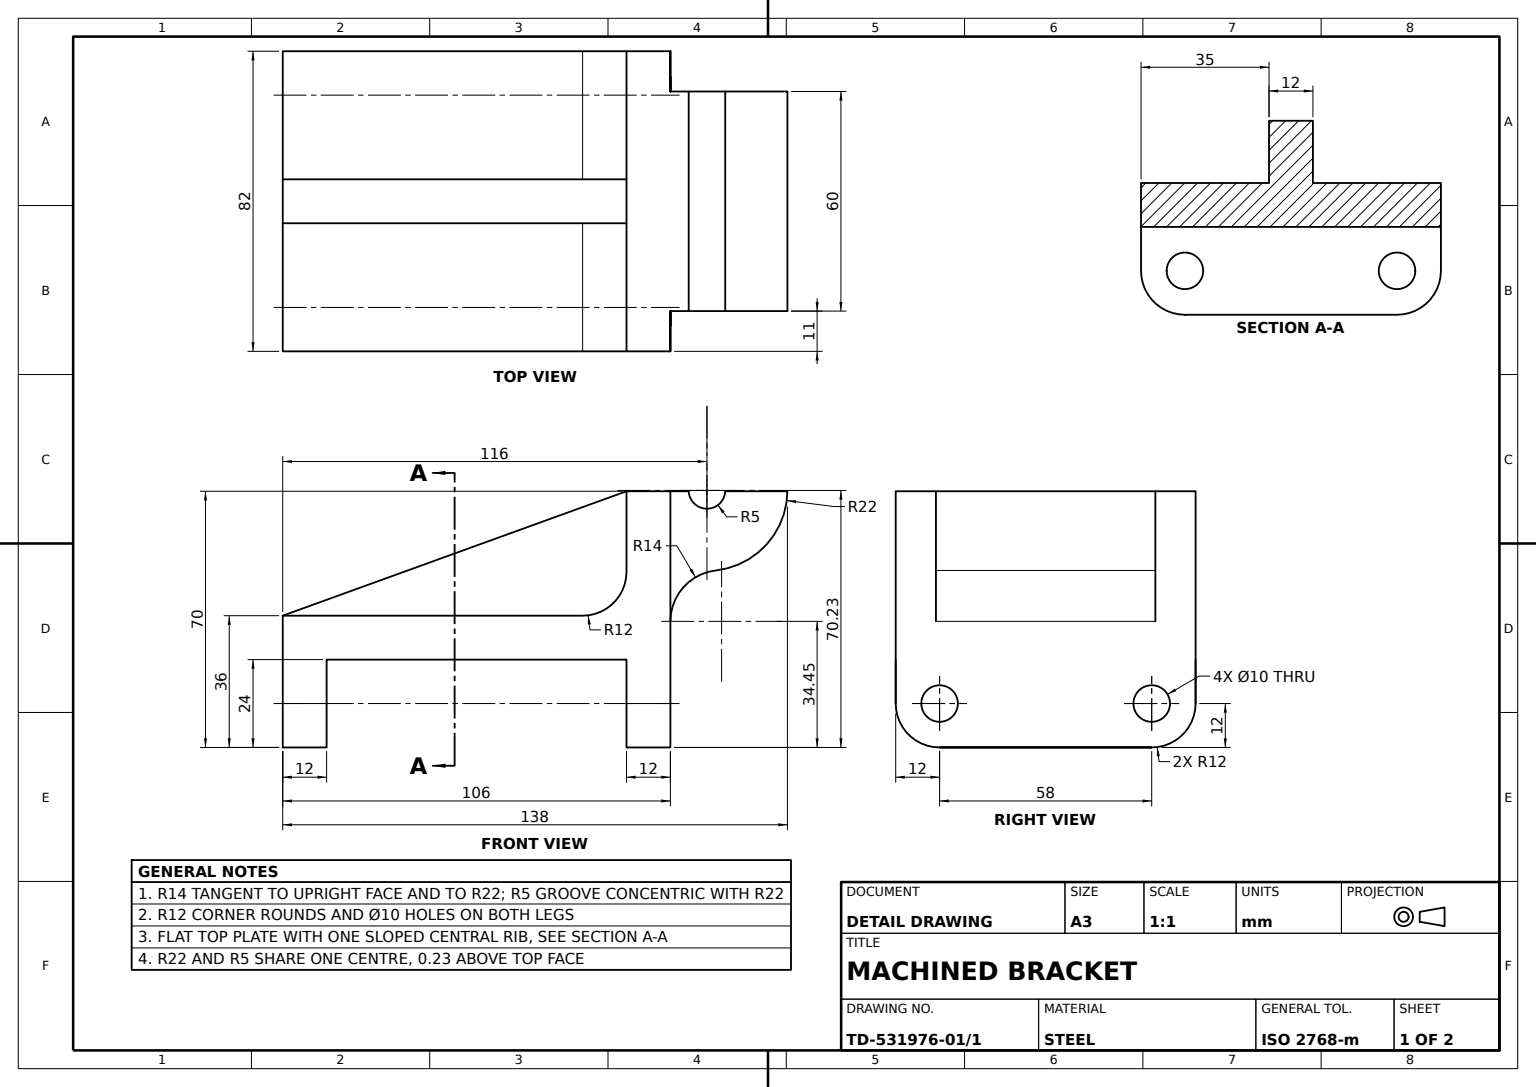
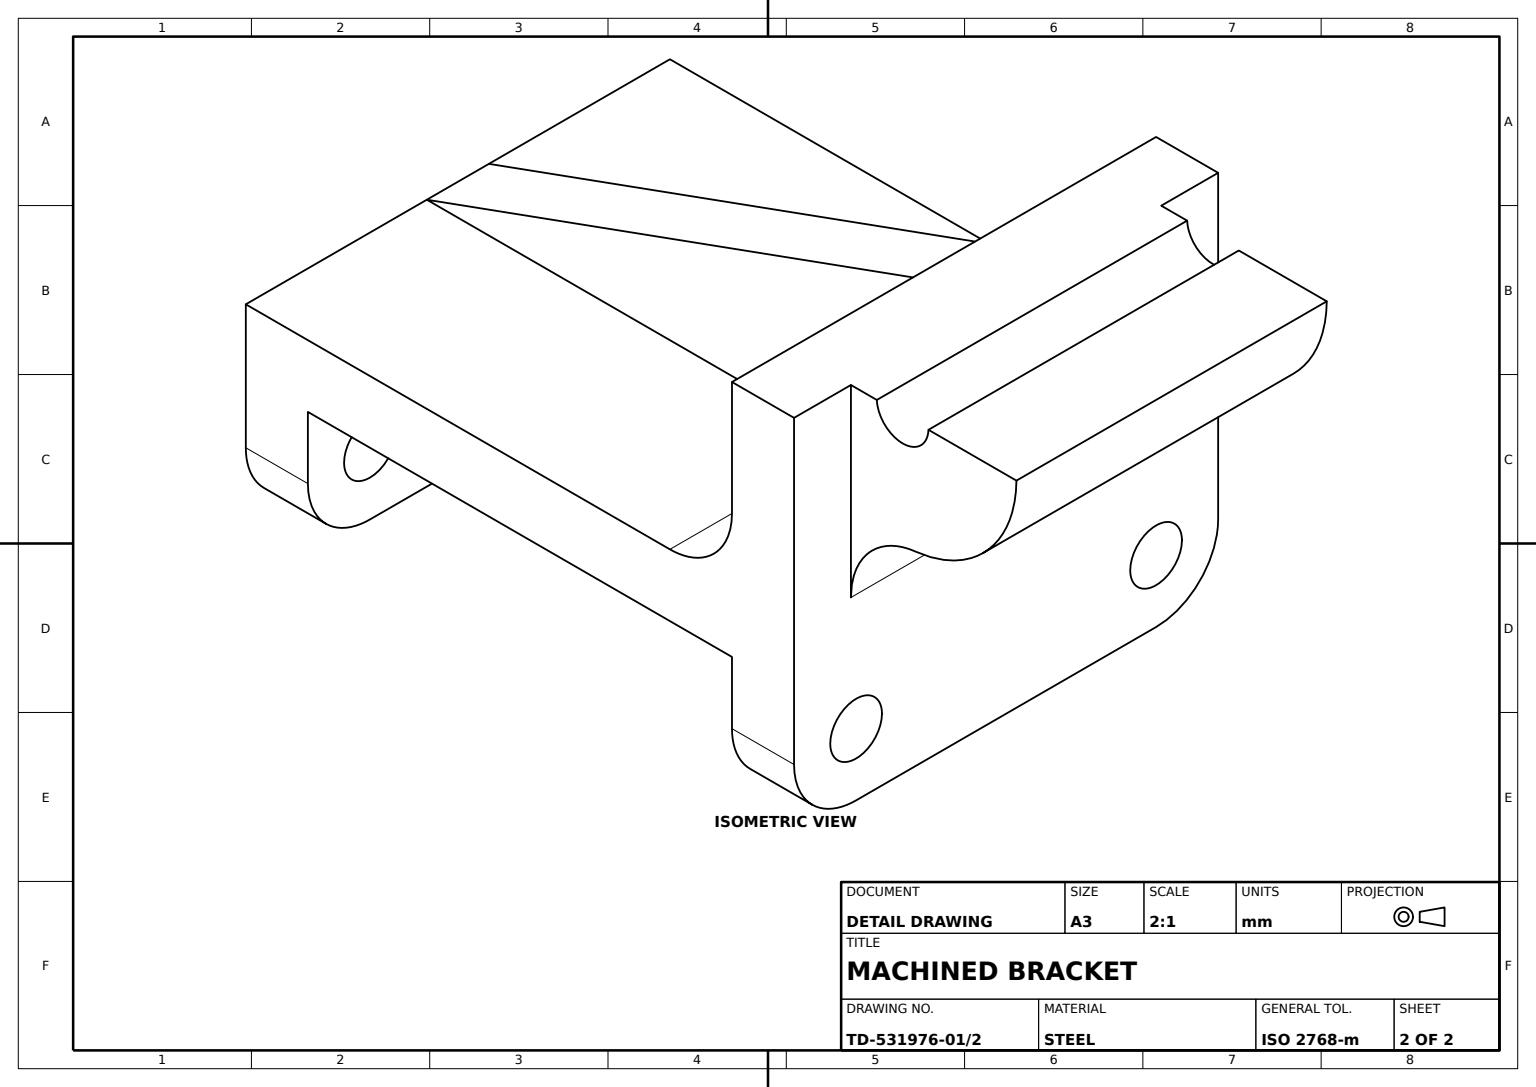
SolidWorks part; units mm, degrees
material "Plain Carbon Steel"
ref_plane "Front Plane" through (0, 0, 0) normal (0, 0, 1) x (1, 0, 0)
ref_plane "Top Plane" through (0, 0, 0) normal (0, 1, 0) x (1, 0, 0)
ref_plane "Right Plane" through (0, 0, 0) normal (1, 0, 0) x (0, 0, -1)
sketch "Bracket Profile Sketch" plane through (0, 0, 0) normal (1, 0, 0) x (0, 0, -1)
  line L0 (0, 0) -> (12, 0)
  line L1 (12, 0) -> (12, 24)
  line L2 (12, 24) -> (94, 24)
  line L3 (94, 24) -> (94, 0)
  line L4 (94, 0) -> (106, 0)
  line L5 (106, 0) -> (106, 70)
  line L6 (106, 70) -> (94, 70)
  line L7 (94, 70) -> (94, 36)
  line L8 (94, 36) -> (0, 36)
  line L9 (0, 36) -> (0, 0)
  dimension "D1" = 106
  dimension "D2" = 82
  dimension "D3" = 12
  dimension "D4" = 70
  dimension "D5" = 24
  dimension "D6" = 36
extrude "Bracket Body" add sketch "Bracket Profile Sketch" along normal blind 82
fillet "Body Corner Fillets R12" radius 12 4 edges at (82, 0, -100) (0, 0, -100) (0, 0, -6) (82, 0, -6)
sketch "Mounting Holes Sketch" plane through (0, 0, 0) normal (0, 0, 1) x (1, 0, 0)
  circle A0 centre (12, 12) radius 5
  circle A1 centre (70, 12) radius 5
  dimension "D1" = 10
  dimension "D2" = 10
extrude "Mounting Holes" cut sketch "Mounting Holes Sketch" against normal through all
ref_plane "Rib Mid Plane" through (41, 0, 0) normal (1, 0, 0) x (0, 0, -1)
sketch "Rib Sketch" plane through (41, 0, 0) normal (1, 0, 0) x (0, 0, -1)
  line L0 (94, 70) -> (0, 36)
rib "Centre Rib 12mm" sketch "Rib Sketch" sketch "Rib Sketch" thickness 12 extrusion direction parallel to sketch draft on no parameters "D1"=12
fillet "Inner Corner Fillet R12" radius 12 2 edges at (17.5, 36, -94) (64.5, 36, -94)
ref_plane "Cradle Sketch Plane" through (41, 0, 0) normal (1, 0, 0) x (0, 0, -1)
sketch "Cradle Profile Sketch" plane through (41, 0, 0) normal (1, 0, 0) x (0, 0, -1)
  line L1 (106, 12) -> (106, 70) construction
  line L2 (120.9949, 70) -> (137.9988, 70)
  line L3 (106, 34.449) -> (106, 70)
  line L4 (106, 70) -> (111.0051, 70)
  arc A0 (137.9988, 70) -> (118.4444, 48.3623) centre (116, 70.2261) cw
  arc A1 (118.4444, 48.3623) -> (106, 34.449) centre (120, 34.449) ccw
  arc A2 (111.0051, 70) -> (120.9949, 70) centre (116, 70.2261) ccw
  dimension "D1" = 22
  dimension "D2" = 10
  dimension "D3" = 10
  dimension "D4" = 14
  dimension "D5" = 34.449
extrude "Cradle Boss" add sketch "Cradle Profile Sketch" along normal mid plane 60
